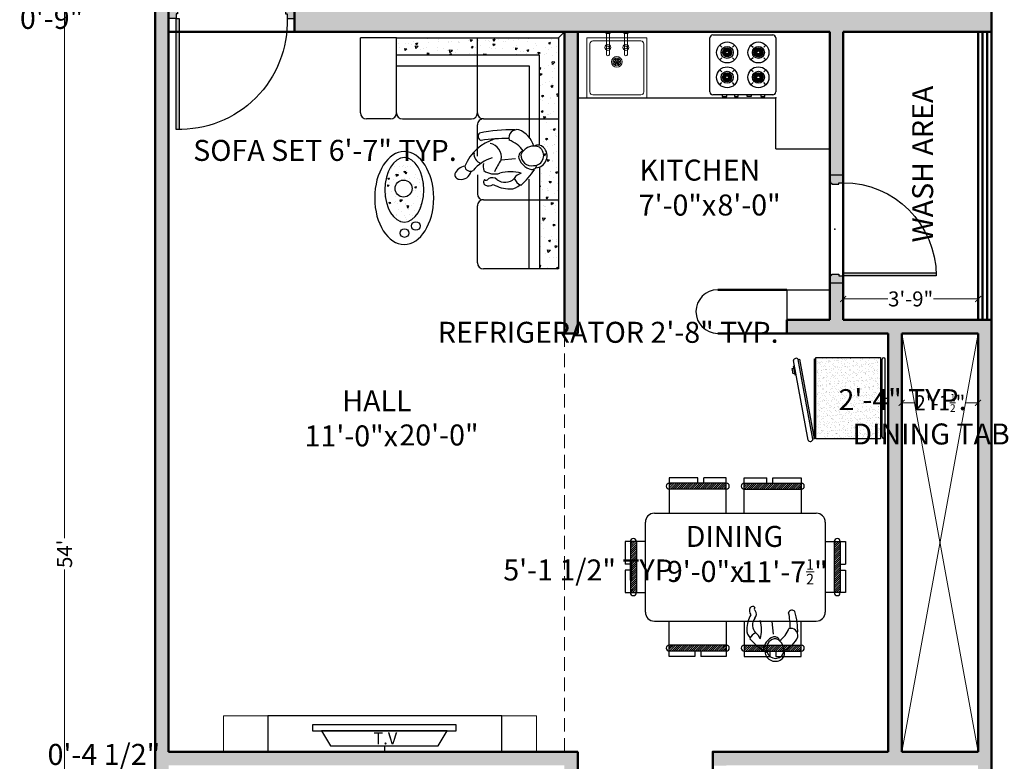
# Model space of a CAD drawing. Units: inches. Extents: x 4508 to 5907, y 877 to 1592.
# Tile 5 of 20: x 4874 to 5203, y 1182 to 1429. Entities that reach past the tile are written whole.
import ezdxf

# ---------------------------------------------------------------- set-up
doc = ezdxf.new("R2010")
doc.units = ezdxf.units.IN
doc.linetypes.add('DASHED', pattern=[0.75, 0.5, -0.25])
doc.layers.get('DEFPOINTS').update_dxf_attribs({"color": 8})
for name, color, linetype, lineweight in [('A-ANNO-DIMS', 2, 'Continuous', 18), ('A-ANNO-TEXT', 7, 'Continuous', 25), ('A-DOOR', 4, 'Continuous', 25), ('A-FLOR-CASE', 30, 'Continuous', 25), ('A-FLOR-FIXT', 8, 'Continuous', 18), ('A-FLOR-OVHD', 5, 'DASHED', 18), ('A-FLOR-SHFT', 8, 'Continuous', 18), ('A-FURN', 24, 'Continuous', 18), ('A-WALL', 7, 'Continuous', 50), ('A-WALL-PATT', 8, 'Continuous', 13)]:
    doc.layers.add(name, color=color, linetype=linetype, lineweight=lineweight)
doc.layers.add('doors & windows', color=30, linetype='Continuous')
doc.layers.add('furniture', color=24, linetype='Continuous')
doc.styles.get("Standard").update_dxf_attribs({"font": 'arial.ttf'})
doc.dimstyles.new('details', dxfattribs={"dimtxt": 5, "dimasz": 2, "dimexe": 2, "dimexo": 3, "dimgap": 1, "dimtad": 0, "dimdec": 1, "dimzin": 0, "dimdsep": 46, "dimlunit": 4, "dimtxsty": 'Standard', "dimblk": 'ARCHTICK', "dimcen": 3, "dimclrd": 256, "dimclre": 256, "dimclrt": 256, "dimadec": 0, "dimazin": 0, "dimtfac": 0.5, "dimtdec": 1, "dimtofl": 0, "dimtmove": 0, "dimatfit": 3, "dimldrblk": 'CLOSEDBLANK', "dimfxl": 2, "dimtolj": 1, "dimtzin": 0, "dimlwd": -1, "dimlwe": -1, "dimarcsym": 0})
doc.dimstyles.new('text', dxfattribs={"dimtxt": 7, "dimasz": 0, "dimexe": 3, "dimexo": 3, "dimgap": 0, "dimtad": 1, "dimtih": 1, "dimtoh": 1, "dimzin": 3, "dimdsep": 46, "dimlunit": 4, "dimtxsty": 'Standard', "dimblk": 'CLOSEDBLANK', "dimcen": 3, "dimse1": 1, "dimse2": 1, "dimsd1": 1, "dimsd2": 1, "dimclrd": 256, "dimclre": 256, "dimclrt": 256, "dimadec": 0, "dimazin": 0, "dimtfac": 0.5, "dimtofl": 0, "dimtmove": 0, "dimatfit": 3, "dimfxl": 3, "dimtolj": 1, "dimtzin": 0, "dimlwd": -1, "dimlwe": -1, "dimarcsym": 0})
pattern_1 = [(45, (0, 0), (-0.3535534, 0.3535534), [])]

# ---------------------------------------------------------------- blocks, each defined once
blk = doc.blocks.new('_ArchTick')
at = {"color": 0, "linetype": 'ByBlock', "const_width": 0.15}
blk.add_lwpolyline([(-0.5, -0.5), (0.5, 0.5)], dxfattribs=at)
blk = doc.blocks.new('*D52')
at = {"layer": 'A-ANNO-DIMS', "color": 0, "transparency": 16777216}
for p, q in [((4877.24, 1574.7), (4891.29, 1574.7)), ((4889.29, 1574.7), (4889.29, 1255.95)), ((4889.29, 926.7), (4889.29, 1245.46)), ((4877.24, 926.7), (4891.29, 926.7))]:
    blk.add_line(p, q, dxfattribs=at)
at = {"layer": 'DEFPOINTS', "color": 0, "transparency": 16777216}
for p in [(4874.24, 1574.7), (4874.24, 926.7), (4889.29, 926.7)]:
    blk.add_point(p, dxfattribs=at)
at = {"layer": 'A-ANNO-DIMS', "color": 0, "transparency": 16777216, "xscale": 2, "yscale": 2, "zscale": 2}
for p, rotation in [((4889.29, 1574.7), 90), ((4889.29, 926.7), 270)]:
    blk.add_blockref('_ArchTick', p, dxfattribs=dict(at, rotation=rotation))
at = {"layer": 'A-ANNO-DIMS', "color": 0, "transparency": 16777216, "insert": (4889.29, 1250.7), "char_height": 5, "attachment_point": 5, "rotation": 90}
blk.add_mtext("\\A1;54'", dxfattribs=at)
blk = doc.blocks.new('_ClosedBlank')
at = {"color": 0, "lineweight": -2}
for p, q in [((-1, 0.17), (0, 0)), ((-1, 0.17), (-1, -0.17)), ((0, 0), (-1, -0.17))]:
    blk.add_line(p, q, dxfattribs=at)
blk = doc.blocks.new('MD')
at = {"layer": 'doors & windows'}
h = blk.add_hatch(dxfattribs=at)
h.set_pattern_fill('DOTS', color=256, scale=2, style=0)
h.set_pattern_definition([(180, (0, -4), (-0.0625, 0.125), [0, -0.125])])
h.paths.add_polyline_path([(2.5, 37), (3.5, 37), (3.5, 0), (2.5, 0)])
h = blk.add_hatch(dxfattribs=at)
h.set_pattern_fill('DOTS', color=256, scale=2, style=0)
h.set_pattern_definition([(0, (0, -0.5), (0.0625, 0.125), [0, -0.125])])
h.paths.add_polyline_path([(42, -4.5), (42, 0), (39.5, 0), (39.5, -1.5), (39, -1.5), (39, -3.75), (39.25, -3.75, 0.403966), (39.75, -4.25), (39.75, -4.5)])
h.paths.add_polyline_path([(0, -4.5), (2.25, -4.5), (2.25, -4.25, 0.403966), (2.75, -3.75), (3, -3.75), (3, -1.5), (2.5, -1.5), (2.5, 0), (0, 0)])
for p, q in [((0, 0), (0, -4.5)), ((42, 0), (42, -4.5))]:
    blk.add_line(p, q)
blk.add_line((0, -4.5), (2.25, -4.5), dxfattribs=at)
blk.add_lwpolyline([(3.5, 0), (3.5, 37), (2.5, 37), (2.5, 0)], close=True, dxfattribs=at)
for points in [[(3, -3.75), (3, -1.5), (2.5, -1.5), (2.5, 0), (0, 0)], [(39, -3.75), (39, -1.5), (39.5, -1.5), (39.5, 0), (42, 0)], [(42, -4.5), (39.75, -4.5)]]:
    blk.add_lwpolyline(points, dxfattribs=at)
for points in [[(2.25, -4.5), (2.25, -4.25, 0.403966), (2.75, -3.75), (3, -3.75)], [(39.75, -4.5), (39.75, -4.25, -0.403966), (39.25, -3.75), (39, -3.75)]]:
    blk.add_lwpolyline(points, format="xyb", dxfattribs=at)
at = {"layer": 'doors & windows', "ltscale": 6}
blk.add_arc((3.73, 1.23), 35.79, 358.0281, 91.9719, dxfattribs=at)
at = {"layer": 'doors & windows'}
blk.add_point((21, -2.75), dxfattribs=at)
blk = doc.blocks.new('*D55')
at = {"layer": 'A-ANNO-DIMS', "color": 0, "transparency": 16777216}
for p, q in [((5148.99, 1331.7), (5148.99, 1337.68)), ((5193.99, 1331.7), (5193.99, 1337.68)), ((5148.99, 1335.68), (5163.85, 1335.68)), ((5193.99, 1335.68), (5179.14, 1335.68))]:
    blk.add_line(p, q, dxfattribs=at)
at = {"layer": 'DEFPOINTS', "color": 0, "transparency": 16777216}
for p in [(5193.99, 1335.68), (5148.99, 1328.7), (5193.99, 1328.7)]:
    blk.add_point(p, dxfattribs=at)
at = {"layer": 'A-ANNO-DIMS', "color": 0, "transparency": 16777216, "xscale": 2, "yscale": 2, "zscale": 2, "rotation": 180}
blk.add_blockref('_ArchTick', (5148.99, 1335.68), dxfattribs=at)
at = {"layer": 'A-ANNO-DIMS', "color": 0, "transparency": 16777216, "xscale": 2, "yscale": 2, "zscale": 2}
blk.add_blockref('_ArchTick', (5193.99, 1335.68), dxfattribs=at)
at = {"layer": 'A-ANNO-DIMS', "color": 0, "transparency": 16777216, "insert": (5171.49, 1335.68), "char_height": 5, "attachment_point": 5}
blk.add_mtext('\\A1;3\'-9"', dxfattribs=at)
blk = doc.blocks.new('D1')
at = {"layer": 'doors & windows'}
h = blk.add_hatch(dxfattribs=at)
h.set_pattern_fill('DOTS', color=256, scale=2, angle=180, style=0)
h.set_pattern_definition([(180, (-2e-12, -4), (-0.0625, -0.125), [0, -0.125])])
h.paths.add_polyline_path([(2.5, 0), (3.5, 0), (3.5, 30.98, 0.008066), (2.5, 31)])
h = blk.add_hatch(dxfattribs=at)
h.set_pattern_fill('DOTS', color=256, scale=2, angle=180, style=0)
h.set_pattern_definition([(180, (0, -0.5), (-0.0625, -0.125), [0, -0.125])])
h.paths.add_polyline_path([(0, -4.5), (2.25, -4.5), (2.25, -4.25, 0.403966), (2.75, -3.75), (3, -3.75), (3, -1.5), (2.5, -1.5), (2.5, 0), (0, 0)])
h.paths.add_polyline_path([(36, -4.5), (36, 0), (33.5, 0), (33.5, -1.5), (33, -1.5), (33, -3.75), (33.25, -3.75, 0.403966), (33.75, -4.25), (33.75, -4.5)])
for p, q in [((0, 0), (0, -4.5)), ((36, 0), (36, -4.5))]:
    blk.add_line(p, q)
blk.add_lwpolyline([(3.5, 0), (3.5, 31), (2.5, 31), (2.5, 0)], close=True, dxfattribs=at)
for points in [[(3, -3.75), (3, -1.5), (2.5, -1.5), (2.5, 0), (0, 0)], [(33, -3.75), (33, -1.5), (33.5, -1.5), (33.5, 0), (36, 0)], [(0, -4.5), (2.25, -4.5)], [(36, -4.5), (33.75, -4.5)]]:
    blk.add_lwpolyline(points, dxfattribs=at)
for points in [[(2.25, -4.5), (2.25, -4.25, 0.403966), (2.75, -3.75), (3, -3.75)], [(33.75, -4.5), (33.75, -4.25, -0.403966), (33.25, -3.75), (33, -3.75)]]:
    blk.add_lwpolyline(points, format="xyb", dxfattribs=at)
at = {"layer": 'doors & windows', "ltscale": 6}
blk.add_arc((2.5, 0), 31, 0, 90, dxfattribs=at)
at = {"layer": 'doors & windows'}
blk.add_point((18, -2.75), dxfattribs=at)
blk = doc.blocks.new('*D56')
at = {"layer": 'DEFPOINTS', "color": 0, "transparency": 16777216}
for p in [(5060.49, 1374.45), (5144.49, 1370.4), (5144.49, 1363.32)]:
    blk.add_point(p, dxfattribs=at)
at = {"layer": 'A-ANNO-DIMS', "color": 0, "transparency": 16777216, "insert": (5093.7, 1372.79), "char_height": 7, "attachment_point": 5}
blk.add_mtext('\\A1;       KITCHEN\\P7\'-0"x', dxfattribs=at)
blk = doc.blocks.new('*D57')
at = {"layer": 'DEFPOINTS', "color": 0, "transparency": 16777216}
for p in [(5099.76, 1424.7), (5117.58, 1424.7), (5125.91, 1328.7)]:
    blk.add_point(p, dxfattribs=at)
at = {"layer": 'A-ANNO-DIMS', "color": 0, "transparency": 16777216, "insert": (5117.58, 1367), "char_height": 7, "attachment_point": 5}
blk.add_mtext('\\A1;8\'-0"', dxfattribs=at)
blk = doc.blocks.new('stove')
at = {"layer": 'furniture'}
h = blk.add_hatch(dxfattribs=at)
h.set_pattern_fill('HEX', color=256, angle=180, style=0)
h.set_pattern_definition([(360, (22, 21.5), (1e-16, 0.2165064), [0.125, -0.25]), (120, (22, 21.5), (-0.1875, -0.1082532), [0.125, -0.25]), (60, (22.125, 21.5), (-0.1875, 0.1082532), [0.125, -0.25])])
h.paths.add_polyline_path([(5.36, 16.21, 1), (8.36, 16.21, 1)])
h.paths.add_polyline_path([(7.36, 16.21, -1), (6.36, 16.21, -1)], flags=16)
h = blk.add_hatch(dxfattribs=at)
h.set_pattern_fill('HEX', color=256, angle=180, style=0)
h.set_pattern_definition([(180, (2e-13, 21.5), (-1e-16, 0.2165064), [0.125, -0.25]), (60, (2e-13, 21.5), (0.1875, -0.1082532), [0.125, -0.25]), (120, (-0.125, 21.5), (0.1875, 0.1082532), [0.125, -0.25])])
h.paths.add_polyline_path([(13.64, 16.21, 1), (16.64, 16.21, 1)])
h.paths.add_polyline_path([(15.64, 16.21, -1), (14.64, 16.21, -1)], flags=16)
h = blk.add_hatch(dxfattribs=at)
h.set_pattern_fill('HEX', color=256, angle=180, style=0)
h.set_pattern_definition([(360, (22, 0.5), (-1e-16, -0.2165064), [0.125, -0.25]), (240, (22, 0.5), (-0.1875, 0.1082532), [0.125, -0.25]), (300, (22.125, 0.5), (-0.1875, -0.1082532), [0.125, -0.25])])
h.paths.add_polyline_path([(8.36, 5.79, 1), (5.36, 5.79, 1)])
h.paths.add_polyline_path([(6.36, 5.79, -1), (7.36, 5.79, -1)], flags=16)
h = blk.add_hatch(dxfattribs=at)
h.set_pattern_fill('HEX', color=256, angle=180, style=0)
h.set_pattern_definition([(180, (2e-13, 0.5), (1e-16, -0.2165064), [0.125, -0.25]), (300, (2e-13, 0.5), (0.1875, 0.1082532), [0.125, -0.25]), (240, (-0.125, 0.5), (0.1875, -0.1082532), [0.125, -0.25])])
h.paths.add_polyline_path([(16.64, 5.79, 1), (13.64, 5.79, 1)])
h.paths.add_polyline_path([(14.64, 5.79, -1), (15.64, 5.79, -1)], flags=16)
for p, q in [((1, 1), (1, 21)), ((2, 22), (20, 22)), ((21, 21), (21, 1)), ((1, 17.86), (0.5, 17.86)), ((0.5, 17.86), (0.5, 16.36)), ((4.39, 18.69), (5.1, 17.98)), ((8.63, 17.98), (9.34, 18.69)), ((13.37, 17.98), (12.66, 18.69)), ((17.61, 18.69), (16.9, 17.98)), ((0.5, 16.36), (1, 16.36)), ((0.5, 13.8), (0.5, 12.5)), ((1, 13.8), (0.5, 13.8)), ((4.39, 13.74), (5.1, 14.45)), ((8.63, 14.45), (9.34, 13.74)), ((13.37, 14.45), (12.66, 13.74)), ((17.61, 13.74), (16.9, 14.45)), ((0.5, 12.5), (1, 12.5)), ((0.5, 9.5), (1, 9.5)), ((0.5, 8.2), (0.5, 9.5)), ((1, 8.2), (0.5, 8.2)), ((4.39, 8.26), (5.1, 7.55)), ((8.63, 7.55), (9.34, 8.26)), ((13.37, 7.55), (12.66, 8.26)), ((17.61, 8.26), (16.9, 7.55)), ((0.5, 4.94), (0.5, 3.64)), ((1, 4.94), (0.5, 4.94)), ((0.5, 3.64), (1, 3.64)), ((4.39, 3.31), (5.1, 4.02)), ((8.63, 4.02), (9.34, 3.31)), ((13.37, 4.02), (12.66, 3.31)), ((17.61, 3.31), (16.9, 4.02)), ((20, 0), (2, 0))]:
    blk.add_line(p, q, dxfattribs=at)
for centre, radius in [((6.86, 16.21), 3.5), ((15.14, 16.21), 3.5), ((6.86, 16.21), 2), ((6.86, 16.21), 1.5), ((6.86, 16.21), 0.5), ((15.14, 16.21), 2), ((15.14, 16.21), 1.5), ((15.14, 16.21), 0.5), ((6.86, 5.79), 3.5), ((6.86, 5.79), 2), ((6.86, 5.79), 1.5), ((15.14, 5.79), 3.5), ((15.14, 5.79), 2), ((15.14, 5.79), 1.5), ((6.86, 5.79), 0.5), ((15.14, 5.79), 0.5)]:
    blk.add_circle(centre, radius, dxfattribs=at)
for centre, start, end in [((2, 21), 90, 180), ((20, 21), 0, 90), ((2, 1), 180, 270), ((20, 1), 270, 0)]:
    blk.add_arc(centre, 1, start, end, dxfattribs=at)
at = {"layer": 'furniture', "ltscale": 9}
blk.add_point((0, 0), dxfattribs=at)
blk = doc.blocks.new('sink')
for p, q in [((0, 0), (-24, 0)), ((0, 0), (0, 0)), ((-22, -3), (-2, -3)), ((-22, -23), (-22, -3)), ((-2, -3), (-2, -23)), ((-21, -21), (-21, -5)), ((-20, -4), (-4, -4)), ((-3, -5), (-3, -21)), ((-0.5, -9.5), (-7.5, -9.5)), ((-0.5, -9.5), (-0.5, -10.5)), ((0, -9), (0, -11)), ((-0.5, -10.5), (-7.5, -10.5)), ((-0.5, -15.5), (-7.5, -15.5)), ((-0.5, -15.5), (-0.5, -16.5)), ((0, -15), (0, -17)), ((-0.5, -16.5), (-7.5, -16.5)), ((-20, -22), (-4, -22)), ((-22, -23), (-2, -23))]:
    blk.add_line(p, q)
for centre, radius in [((-5.18, -10), 1), ((-5.18, -10), 0.5), ((-10, -13), 1.79), ((-10, -13), 1.29), ((-10.66, -12.62), 0.25), ((-10.66, -13.38), 0.25), ((-10, -12.24), 0.25), ((-10, -13), 0.25), ((-9.34, -12.62), 0.25), ((-9.34, -13.38), 0.25), ((-10, -13.76), 0.25), ((-5.18, -16), 1), ((-5.18, -16), 0.5)]:
    blk.add_circle(centre, radius)
for centre, radius, start, end in [((-20, -5), 1, 90, 180), ((-4, -5), 1, 0, 90), ((-7.5, -10), 0.5, 90, 270), ((0.01, -9.51), 0.511, 91.1728, 178.8272), ((0.01, -10.49), 0.511, 181.1728, 268.8272), ((-7.5, -16), 0.5, 90, 270), ((0.01, -15.51), 0.511, 91.1728, 178.8272), ((0.01, -16.49), 0.511, 181.1728, 268.8272), ((-20, -21), 1, 180, 270), ((-4, -21), 1, 270, 0)]:
    blk.add_arc(centre, radius, start, end)
blk = doc.blocks.new('*D58')
at = {"layer": 'A-ANNO-DIMS', "color": 0, "transparency": 16777216}
for p, q in [((5168.49, 1321.2), (5168.49, 1299.04)), ((5193.99, 1321.2), (5193.99, 1299.04)), ((5168.49, 1301.04), (5172.64, 1301.04)), ((5193.99, 1301.04), (5189.84, 1301.04))]:
    blk.add_line(p, q, dxfattribs=at)
at = {"layer": 'DEFPOINTS', "color": 0, "transparency": 16777216}
for p in [(5168.49, 1324.2), (5193.99, 1324.2), (5193.99, 1301.04)]:
    blk.add_point(p, dxfattribs=at)
at = {"layer": 'A-ANNO-DIMS', "color": 0, "transparency": 16777216, "xscale": 2, "yscale": 2, "zscale": 2, "rotation": 180}
blk.add_blockref('_ArchTick', (5168.49, 1301.04), dxfattribs=at)
at = {"layer": 'A-ANNO-DIMS', "color": 0, "transparency": 16777216, "xscale": 2, "yscale": 2, "zscale": 2}
blk.add_blockref('_ArchTick', (5193.99, 1301.04), dxfattribs=at)
at = {"layer": 'A-ANNO-DIMS', "color": 0, "transparency": 16777216, "insert": (5181.24, 1301.04), "char_height": 5, "attachment_point": 5}
blk.add_mtext('\\A1;2\'-1{\\H0.5x;\\S1/2;}"', dxfattribs=at)
blk = doc.blocks.new('refrigerator')
at = {"layer": 'furniture'}
h = blk.add_hatch(dxfattribs=at)
h.set_pattern_fill('AR-SAND', color=256, angle=-90, style=0)
h.set_pattern_definition([(307.5, (-13.5104, -1), (1.926824, 0.06299), [0, -1.52, 0, -1.7, 0, -1.625]), (277.5, (-13.5104, -1), (2.82215, -1.76978), [0, -0.82, 0, -1.37, 0, -0.525]), (237.5, (-13.5104, 0.23), (0.00566, -3.11414), [0, -0.5, 0, -1.8, 0, -2.35]), (227.5, (-13.5104, 0.23), (0.87768, -3.00613), [0, -0.25, 0, -1.18, 0, -1.35])])
h.paths.add_polyline_path([(13.6, -24.16), (13.6, -2.56), (-13.51, -2.56), (-13.51, -24.16)])
for p, q in [((0, -1), (0, 0)), ((-13.51, -2.56), (13.6, -2.56)), ((-13.51, -24.16), (-13.51, -2.56)), ((12.94, -1), (-12.94, -1)), ((12.94, -2), (-12.94, -2)), ((-12.41, -2), (-12.41, -2.56)), ((12.29, -2), (12.29, -2.56)), ((13.6, -2.56), (13.6, -24.16)), ((13.6, -24.16), (-13.51, -24.16)), ((-13.07, -24.59), (-13.07, -24.16)), ((13.26, -24.59), (-13.07, -24.59)), ((13.6, -24.61), (-12.95, -29.5)), ((13.7, -25.1), (-12.85, -29.99)), ((13.07, -24.59), (13.26, -24.62)), ((13.26, -24.62), (13.07, -24.71)), ((13.26, -24.59), (13.26, -24.16)), ((13.6, -24.61), (13.7, -25.1)), ((-12.85, -29.99), (-12.95, -29.5)), ((14.06, -26.73), (-12.49, -31.62)), ((-10.58, -31.27), (-10.49, -31.65)), ((-10.49, -31.65), (-7.79, -31.16)), ((-9.87, -32.01), (-9.97, -31.56)), ((-8.13, -31.69), (-9.87, -32.01)), ((-8.23, -31.24), (-8.13, -31.69)), ((-7.79, -31.16), (-7.88, -30.77))]:
    blk.add_line(p, q, dxfattribs=at)
for centre, radius, start, end in [((-12.94, -1.5), 0.5, 90, 270), ((12.94, -1.5), 0.5, 270, 90), ((13.58, -25.98), 0.888, 302.2332, 82.2568), ((-12.38, -30.74), 0.888, 122.2332, 262.2568)]:
    blk.add_arc(centre, radius, start, end, dxfattribs=at)
blk = doc.blocks.new('*D59')
at = {"layer": 'DEFPOINTS', "color": 0, "transparency": 16777216}
for p in [(5055.99, 1241.2), (5163.99, 1238.74), (5055.99, 1237.03)]:
    blk.add_point(p, dxfattribs=at)
at = {"layer": 'A-ANNO-DIMS', "color": 0, "transparency": 16777216, "insert": (5103.1, 1250.67), "char_height": 7, "attachment_point": 5}
blk.add_mtext('\\A1;         DINING\\P9\'-0"x', dxfattribs=at)
blk = doc.blocks.new('*D60')
at = {"layer": 'DEFPOINTS', "color": 0, "transparency": 16777216}
for p in [(5129.27, 1324.2), (5130.19, 1324.2), (5055.99, 1184.7)]:
    blk.add_point(p, dxfattribs=at)
at = {"layer": 'A-ANNO-DIMS', "color": 0, "transparency": 16777216, "insert": (5129.27, 1244.72), "char_height": 7, "attachment_point": 5}
blk.add_mtext('\\A1;11\'-7{\\H0.5x;\\S1/2;}"', dxfattribs=at)
blk = doc.blocks.new('DT')
at = {"layer": 'furniture'}
h = blk.add_hatch(dxfattribs=at)
h.set_pattern_fill('ANSI31', color=256, scale=4, style=0)
h.set_pattern_definition(pattern_1)
h.paths.add_polyline_path([(-34, -8.5), (-32, -8.5), (-32, 8.5), (-34, 8.5)])
h.paths.add_polyline_path([(-2, 26), (-2, 28), (-21, 28), (-21, 26)])
h.paths.add_polyline_path([(23, 26), (23, 28), (4, 28), (4, 26)])
h.paths.add_polyline_path([(23, -28), (23, -26), (4, -26), (4, -28)])
h.paths.add_polyline_path([(-2, -28), (-2, -26), (-21, -26), (-21, -28)])
h = blk.add_hatch(dxfattribs=at)
h.set_pattern_fill('ANSI31', color=256, scale=4, style=0)
h.set_pattern_definition(pattern_1)
h.paths.add_polyline_path([(34, -8.5), (36, -8.5), (36, 8.5), (34, 8.5)])
at = {"layer": 'doors & windows'}
blk.add_line((-11.2, 18.15), (-11.59, 22.33), dxfattribs=at)
for centre, radius, start, end in [((-13.21, 28.75), 2.25, 132.7993, 210.1219), ((-12.43, 27.51), 2.91, 359.7942, 144.0351), ((-12.34, 27.96), 3.42, 2.8928, 134.5528), ((-12.78, 20.33), 7.67, 108.0153, 157.5724), ((-11.2, 27.56), 3.95, 155.2349, 248.5051), ((-12.53, 26.93), 3.05, 267.7788, 10.6507), ((-13.37, 28.03), 5.08, 289.2819, 356.6237), ((-9.72, 27.09), 1.31, 352.7443, 87.7525), ((-20.97, 8.73), 22.84, 41.647, 56.3067), ((-17.49, 22.83), 2.42, 170.002, 284.7527), ((-8.5, 17.23), 8.99, 125.6851, 158.6987), ((-12.08, 24.9), 1.7, 192.3382, 283.0231), ((2.64, 20.82), 10.42, 162.7002, 196.7262), ((-4.27, 24.65), 3.12, 193.5598, 239.9446), ((-6.9, 24.92), 3.16, 289.6374, 341.2911), ((-6.62, 20.83), 3.81, 358.2671, 46.939), ((1.32, 21.08), 21.14, 177.1977, 197.248), ((6.61, 20.49), 23.98, 180.1725, 192.6992), ((-8.79, 19.27), 4.03, 325.4363, 41.8446), ((-13.17, 20.91), 10.36, 330.7562, 358.8997), ((-4.02, 15.59), 2.01, 136.0875, 215.1077), ((-17.93, 15.53), 1.19, 217.214, 345.0614), ((-5.98, 13.86), 0.655, 315.9836, 61.7947), ((-4.79, 14.1), 0.998, 224.0636, 323.687), ((-5.73, 14.57), 2.04, 328.4119, 38.6474)]:
    blk.add_arc(centre, radius, start, end, dxfattribs=at)
at = {"layer": 'furniture'}
for p, q in [((-21, 29.75), (-21, 18)), ((-12.5, 29.75), (-21, 29.75)), ((-12.5, 28), (-12.5, 29.75)), ((-10.5, 28), (-10.5, 29.75)), ((-2, 29.75), (-10.5, 29.75)), ((-2, 18), (-2, 29.75)), ((4, 18), (4, 29.75)), ((4, 29.75), (12.5, 29.75)), ((12.5, 28), (12.5, 29.75)), ((14.5, 28), (14.5, 29.75)), ((14.5, 29.75), (23, 29.75)), ((23, 29.75), (23, 18)), ((-2, 28), (-21, 28)), ((4, 28), (23, 28)), ((-2, 26), (-21, 26)), ((4, 26), (23, 26)), ((28, 18), (-26, 18)), ((-29, -15), (-29, 15)), ((31, 15), (31, -15)), ((-35.75, 1), (-35.75, 8.5)), ((-35.75, 8.5), (-29, 8.5)), ((-34, -8.5), (-34, 8.5)), ((-32, -8.5), (-32, 8.5)), ((37.75, 8.5), (31, 8.5)), ((34, -8.5), (34, 8.5)), ((36, -8.5), (36, 8.5)), ((37.75, 1), (37.75, 8.5)), ((-34, 1), (-35.75, 1)), ((36, 1), (37.75, 1)), ((-34, -1), (-35.75, -1)), ((-35.75, -8.5), (-35.75, -1)), ((36, -1), (37.75, -1)), ((37.75, -8.5), (37.75, -1)), ((-29, -8.5), (-35.75, -8.5)), ((31, -8.5), (37.75, -8.5)), ((28, -18), (-26, -18)), ((-21, -29.75), (-21, -18)), ((-2, -18), (-2, -29.75)), ((4, -18), (4, -29.75)), ((23, -29.75), (23, -18)), ((-2, -26), (-21, -26)), ((4, -26), (23, -26)), ((-2, -28), (-21, -28)), ((-11.5, -28), (-11.5, -29.75)), ((-9.5, -28), (-9.5, -29.75)), ((4, -28), (23, -28)), ((11.5, -28), (11.5, -29.75)), ((13.5, -28), (13.5, -29.75)), ((-11.5, -29.75), (-21, -29.75)), ((-2, -29.75), (-9.5, -29.75)), ((4, -29.75), (11.5, -29.75)), ((13.5, -29.75), (23, -29.75))]:
    blk.add_line(p, q, dxfattribs=at)
for centre, radius, start, end in [((-21, 27), 1, 90, 270), ((-2, 27), 1, 270, 90), ((4, 27), 1, 90, 270), ((23, 27), 1, 270, 90), ((-26, 15), 3, 90, 180), ((28, 15), 3, 0, 90), ((-33, 8.5), 1, 0, 180), ((35, 8.5), 1, 0, 180), ((-33, -8.5), 1, 180, 0), ((35, -8.5), 1, 180, 0), ((-26, -15), 3, 180, 270), ((28, -15), 3, 270, 0), ((-21, -27), 1, 90, 270), ((-2, -27), 1, 270, 90), ((4, -27), 1, 90, 270), ((23, -27), 1, 270, 90)]:
    blk.add_arc(centre, radius, start, end, dxfattribs=at)
blk.add_point((1, 0), dxfattribs=at)
blk = doc.blocks.new('tv')
at = {"layer": 'furniture'}
blk.add_line((0, 0), (2, 0), dxfattribs=at)
for points in [[(0, -39), (12, -39), (12, 39), (0, 39)], [(7, 24.19), (7, -23.81), (9, -23.81), (9, 24.19), (7, 24.19)]]:
    blk.add_lwpolyline(points, dxfattribs=at)
blk.add_lwpolyline([(7, -20.81), (7, 21.19), (2, 18.19), (2, -17.81)], close=True, dxfattribs=at)
blk.add_text('T.V', height=4, rotation=270, dxfattribs=at).set_placement((2.46, 3.81))
blk = doc.blocks.new('MAN')
at = {"layer": 'doors & windows'}
blk.add_line((1.3, -9.85), (0.89, -5.45), dxfattribs=at)
for centre, radius, start, end in [((-0.81, 1.3), 2.37, 132.7993, 210.1219), ((0, 0), 3.06, 359.7942, 144.0351), ((0.1, 0.48), 3.6, 2.8928, 134.5528), ((-0.36, -7.56), 8.07, 108.0153, 157.5724), ((1.3, 0.05), 4.16, 155.2349, 248.5051), ((-0.98, 0.55), 5.34, 289.2819, 356.6237), ((2.86, -0.44), 1.38, 352.7443, 87.7525), ((-8.99, -19.77), 24.04, 41.647, 56.3067), ((-0.1, -0.61), 3.22, 267.7788, 10.6507), ((-5.32, -4.92), 2.54, 170.002, 284.7527), ((34.75, -7.19), 42.53, 177.9613, 192.4551), ((4.14, -10.82), 9.46, 125.6851, 158.6987), ((0.38, -2.75), 1.79, 192.3382, 283.0231), ((15.87, -7.04), 10.97, 162.7002, 196.7262), ((8.59, -3.01), 3.29, 193.5598, 239.9446), ((5.83, -2.73), 3.32, 289.6374, 341.2911), ((3.84, -8.67), 4.24, 325.4363, 41.8446), ((6.12, -7.03), 4.01, 358.2671, 46.939), ((54.76, -7.35), 59.95, 180.1044, 188.2297), ((-0.78, -6.94), 10.91, 330.7562, 358.8997), ((9.03, -7.36), 14.72, 197.1765, 246.7641), ((0.5, -14.05), 4.27, 79.2575, 168.509), ((16.49, 13.41), 27.78, 236.8487, 245.427), ((-0.19, -11.81), 5.78, 325.2412, 16.1794), ((8.85, -12.54), 2.12, 136.0875, 215.1077), ((12.84, -8.62), 12.77, 197.9012, 229.3504), ((6.8, -14.37), 0.689, 315.9836, 61.7947), ((8.05, -14.12), 1.05, 224.0636, 323.687), ((7.06, -13.61), 2.15, 328.4119, 38.6474), ((-5.78, -15.61), 1.25, 217.214, 345.0614), ((-0.4, -15.27), 2.81, 261.6005, 345.5998), ((3.21, -8.72), 6.53, 262.8142, 281.931), ((3.09, -19.2), 1.68, 274.444, 31.8659), ((6.99, -20.36), 3.8, 187.9766, 248.0432), ((4.09, -22.01), 3.16, 349.15, 77.9716), ((5.75, -22.44), 1.45, 262.6631, 353.5986)]:
    blk.add_arc(centre, radius, start, end, dxfattribs=at)
blk = doc.blocks.new('sofa 3')
at = {"layer": 'furniture', "ltscale": 0.5}
h = blk.add_hatch(dxfattribs=at)
h.set_pattern_fill('AR-CONC', color=256, angle=90, style=0)
h.set_pattern_definition([(220, (1099.1507, -871.655), (0.627521, -7.172602), [0.75, -8.25]), (275, (1099.151, -871.655), (-7.52192, 1.387513), [0.6, -6.6]), (169.5486, (1099.203, -872.253), (-6.894395, -5.785094), [0.637402, -7.01142]), (223.8158, (1097.151, -871.655), (1.65519, -10.67241), [1.125, -12.375]), (173.3644, (1097.289, -872.544), (-9.74118, -9.34663), [0.9561, -10.51713]), (278.8158, (1097.151, -871.655), (-9.74119, -9.34662), [0.9, -9.9]), (249, (1097.6507, -872.655), (4.02619, -5.96907), [0.75, -8.25]), (304, (1097.651, -872.655), (-7.2515, -2.433153), [0.6, -6.6]), (198.5486, (1097.986, -873.1524), (-3.225305, -8.402226), [0.637402, -7.01142]), (232.5, (1099.1507, -871.655), (-3.3289385, -0.1215986), [0, -6.52, 0, -6.7, 0, -6.625]), (262.5, (1099.1507, -871.655), (-3.944117, -2.630695), [0, -3.82, 0, -6.37, 0, -2.525]), (302.5, (1099.1507, -869.425), (0.2255487, -5.3382244), [0, -2.5, 0, -7.8, 0, -10.35]), (312.5, (1099.1507, -868.425), (-1.00105, -5.831862), [0, -3.25, 0, -5.18, 0, -7.35])])
h.paths.add_polyline_path([(2, 56), (2, 79), (8.27, 79), (8.27, 56)])
edge = h.paths.add_edge_path()
edge.add_arc((9.44, 36.7), 1.54, 139.4115, 177.7525)
edge.add_arc((8.94, 33.52), 3.4, 107.8673, 234.0351)
edge.add_arc((8.88, 34.97), 4.62, 245.2349, 262.3616)
edge.add_line((8.27, 30.38), (8.27, 29))
edge.add_line((8.27, 29), (2, 29))
edge.add_line((2, 29), (2, 56))
edge.add_line((2, 56), (8.27, 56))
edge.add_line((8.27, 56), (8.27, 37.7))
h.paths.add_polyline_path([(8.27, 7.77), (29, 7.77), (29, 2), (2, 2), (2, 29), (8.27, 29)])
h.paths.add_polyline_path([(29, 2), (29, 7.77), (56, 7.77), (56, 2)])
at = {"layer": 'furniture'}
h = blk.add_hatch(dxfattribs=at)
h.set_pattern_fill('AR-CONC', color=256, scale=0.8, angle=90, style=0)
h.set_pattern_definition([(220, (892.888, -686.9864), (0.502017, -5.738081), [0.6, -6.6]), (275, (892.888, -686.9864), (-6.017537, 1.11001), [0.48, -5.28]), (169.5486, (892.93, -687.4646), (-5.515516, -4.628075), [0.509922, -5.609137]), (223.8158, (891.288, -686.9864), (1.32415, -8.53793), [0.9, -9.9]), (173.3644, (891.3985, -687.698), (-7.79294, -7.4773), [0.76488, -8.413704]), (278.8158, (891.288, -686.986), (-7.79295, -7.477296), [0.72, -7.92]), (249, (891.688, -687.7864), (3.220951, -4.775256), [0.6, -6.6]), (304, (891.688, -687.7864), (-5.8012, -1.946523), [0.48, -5.28]), (198.5486, (891.9566, -688.1844), (-2.580244, -6.72178), [0.509922, -5.609137]), (232.5, (892.8881, -686.9864), (-2.663151, -0.097279), [0, -5.216, 0, -5.36, 0, -5.3]), (262.5, (892.8881, -686.9864), (-3.155294, -2.104556), [0, -3.056, 0, -5.096, 0, -2.02]), (302.5, (892.8881, -685.2024), (0.180439, -4.2705795), [0, -2, 0, -6.24, 0, -8.28]), (312.5, (892.888, -684.4024), (-0.80084, -4.665489), [0, -2.6, 0, -4.144, 0, -5.88])])
edge = h.paths.add_edge_path()
edge.add_ellipse((53.37, 52.67), major_axis=(0, 10.76), ratio=0.60396, start_angle=0, end_angle=360, ccw=False)
h.paths.add_polyline_path([(56.46, 52.22, -1), (50.81, 52.22, -1)], flags=16)
for p, q in [((2, 2), (2, 79)), ((2, 79), (27, 79)), ((8.27, 44.99), (8.27, 79)), ((11.8, 79), (11.8, 49.12)), ((29, 77), (29, 58)), ((27, 56), (2, 56)), ((29, 47.65), (29, 54)), ((29, 41.41), (29, 31)), ((8.27, 37.77), (8.27, 7.77)), ((11.8, 11.29), (11.8, 35.08)), ((8.27, 29), (2, 29)), ((27, 29), (8.27, 29)), ((29, 27), (29, 2)), ((54, 29), (31, 29)), ((56, 27), (56, 2)), ((58, 29), (66, 29)), ((68, 27), (68, 2)), ((56, 11.29), (11.8, 11.29)), ((8.27, 7.77), (56, 7.77)), ((2, 2), (0, 0)), ((56, 2), (2, 2)), ((56, 2), (68, 2))]:
    blk.add_line(p, q, dxfattribs=at)
for centre, radius in [((49.58, 64.71), 1.44), ((53.36, 67.05), 1.44), ((53.63, 52.22), 2.83)]:
    blk.add_circle(centre, radius, dxfattribs=at)
for centre, start, end in [((27, 77), 0, 90), ((27, 58), 270, 0), ((27, 54), 0, 90), ((27, 31), 270, 0), ((27, 27), 0, 90), ((31, 27), 90, 180), ((54, 27), 0, 90), ((58, 27), 90, 180), ((66, 27), 0, 90)]:
    blk.add_arc(centre, 2, start, end, dxfattribs=at)
at = {"layer": 'furniture', "extrusion": (0, 0, -1)}
for centre, major_axis, ratio in [((53.43, 55.37), (0, 15.49), 0.635514), ((53.37, 52.67), (0, 10.76), 0.60396)]:
    blk.add_ellipse(centre, major_axis=major_axis, ratio=ratio, dxfattribs=at)
at = {"xscale": 1.1, "yscale": 1.1, "zscale": 1.1, "rotation": 90}
blk.add_blockref('MAN', (10.27, 41.21), dxfattribs=at)
blk = doc.blocks.new('*D71')
at = {"layer": 'DEFPOINTS', "color": 0, "transparency": 16777216}
for p in [(5002.43, 1422.87), (5014.16, 1422.87), (4995.88, 1182.87)]:
    blk.add_point(p, dxfattribs=at)
at = {"layer": 'A-ANNO-DIMS', "color": 0, "transparency": 16777216, "insert": (5014.16, 1290.32), "char_height": 7, "attachment_point": 5}
blk.add_mtext('\\A1;20\'-0"', dxfattribs=at)
blk = doc.blocks.new('*D72')
at = {"layer": 'DEFPOINTS', "color": 0, "transparency": 16777216}
for p in [(5063.81, 1286.44), (5063.81, 1261.14), (4931.81, 1252.3)]:
    blk.add_point(p, dxfattribs=at)
at = {"layer": 'A-ANNO-DIMS', "color": 0, "transparency": 16777216, "insert": (4984.91, 1295.85), "char_height": 7, "attachment_point": 5}
blk.add_mtext('\\A1;        HALL\\P11\'-0"x', dxfattribs=at)
blk = doc.blocks.new('*D77')
at = {"layer": 'A-ANNO-DIMS', "color": 0, "transparency": 16777216}
for p, q in [((5201.49, 1574.7), (5213.97, 1574.7)), ((5211.97, 1574.7), (5211.97, 1255.95)), ((5211.97, 926.7), (5211.97, 1245.46)), ((5201.49, 926.7), (5213.97, 926.7))]:
    blk.add_line(p, q, dxfattribs=at)
at = {"layer": 'DEFPOINTS', "color": 0, "transparency": 16777216}
for p in [(5198.49, 1574.7), (5211.97, 1574.7), (5198.49, 926.7)]:
    blk.add_point(p, dxfattribs=at)
at = {"layer": 'A-ANNO-DIMS', "color": 0, "transparency": 16777216, "xscale": 2, "yscale": 2, "zscale": 2}
for p, rotation in [((5211.97, 1574.7), 90), ((5211.97, 926.7), 270)]:
    blk.add_blockref('_ArchTick', p, dxfattribs=dict(at, rotation=rotation))
at = {"layer": 'A-ANNO-DIMS', "color": 0, "transparency": 16777216, "insert": (5211.97, 1250.7), "char_height": 5, "attachment_point": 5, "rotation": 90}
blk.add_mtext("\\A1;54'", dxfattribs=at)
blk = doc.blocks.new('*D168')
at = {"layer": 'DEFPOINTS', "color": 0, "transparency": 16777216}
for p in [(5163.99, 1320.93), (5131.98, 1316.12), (5163.99, 1316.12)]:
    blk.add_point(p, dxfattribs=at)
at = {"layer": 'A-ANNO-DIMS', "transparency": 16777216, "insert": (5070.62, 1324.55), "char_height": 7, "attachment_point": 5}
blk.add_mtext('\\A1;REFRIGERATOR 2\'-8" TYP.', dxfattribs=at)
blk = doc.blocks.new('*D169')
at = {"layer": 'DEFPOINTS', "color": 0, "transparency": 16777216}
for p in [(5163.99, 1316.12), (5163.99, 1288.08), (5168.79, 1288.08)]:
    blk.add_point(p, dxfattribs=at)
at = {"layer": 'A-ANNO-DIMS', "transparency": 16777216, "insert": (5168.79, 1302.1), "char_height": 7, "attachment_point": 5}
blk.add_mtext('\\A1;2\'-4" TYP.', dxfattribs=at)
blk = doc.blocks.new('*D170')
at = {"layer": 'DEFPOINTS', "color": 0, "transparency": 16777216}
for p in [(4987.99, 1424.7), (4976.14, 1345.7), (4987.99, 1345.7)]:
    blk.add_point(p, dxfattribs=at)
at = {"layer": 'A-ANNO-DIMS', "transparency": 16777216, "insert": (4976.14, 1385.2), "char_height": 7, "attachment_point": 5}
blk.add_mtext('\\A1;SOFA SET 6\'-7" TYP.', dxfattribs=at)
blk = doc.blocks.new('*D171')
at = {"layer": 'DEFPOINTS', "color": 0, "transparency": 16777216}
for p in [(4987.99, 1436.55), (4987.99, 1424.7), (5055.99, 1424.7)]:
    blk.add_point(p, dxfattribs=at)
at = {"layer": 'A-ANNO-DIMS', "transparency": 16777216, "insert": (5021.99, 1440.13), "char_height": 7, "attachment_point": 5}
blk.add_mtext('\\A1;5\'-8" TYP.', dxfattribs=at)
blk = doc.blocks.new('*D172')
at = {"layer": 'DEFPOINTS', "color": 0, "transparency": 16777216}
for p in [(5076.25, 1287.03), (5076.25, 1276.01), (5149.75, 1276.01)]:
    blk.add_point(p, dxfattribs=at)
at = {"layer": 'A-ANNO-DIMS', "transparency": 16777216, "insert": (5214.38, 1290.65), "char_height": 7, "attachment_point": 5}
blk.add_mtext('\\A1;DINING TABLE 6\'-1 1/2" TYP.', dxfattribs=at)
blk = doc.blocks.new('*D173')
at = {"layer": 'DEFPOINTS', "color": 0, "transparency": 16777216}
for p in [(5076.25, 1276.01), (5065.22, 1214.63), (5076.25, 1214.63)]:
    blk.add_point(p, dxfattribs=at)
at = {"layer": 'A-ANNO-DIMS', "transparency": 16777216, "insert": (5065.22, 1245.32), "char_height": 7, "attachment_point": 5}
blk.add_mtext('\\A1;5\'-1 1/2" TYP.', dxfattribs=at)
blk = doc.blocks.new('*D185')
at = {"layer": 'DEFPOINTS', "color": 0, "transparency": 16777216}
for p in [(4884.941772, 1433.703772), (4923.991772, 1433.703772), (4923.991772, 1424.703772)]:
    blk.add_point(p, dxfattribs=at)
at = {"layer": 'A-ANNO-DIMS', "transparency": 16777216, "insert": (4884.941772, 1429.203772), "char_height": 7, "attachment_point": 5}
blk.add_mtext('\\A1;0\'-9"', dxfattribs=at)
blk = doc.blocks.new('*D187')
at = {"layer": 'DEFPOINTS', "color": 0, "transparency": 16777216}
for p in [(4884.94, 1184.7), (4923.99, 1184.7), (4923.99, 1180.2)]:
    blk.add_point(p, dxfattribs=at)
at = {"layer": 'A-ANNO-DIMS', "transparency": 16777216, "insert": (4902.4, 1183.82), "char_height": 7, "attachment_point": 5}
blk.add_mtext('\\A1;0\'-4 1/2"', dxfattribs=at)

msp = doc.modelspace()

# ---------------------------------------------------------------- hatches: boundary and pattern name
at = {"layer": 'A-WALL-PATT'}
h = msp.add_hatch(color=256, dxfattribs=at)
h.dxf.hatch_style = 1
h.paths.add_polyline_path([(5198.492, 1496.704), (5108.492, 1496.704), (5108.492, 1473.841), (5117.492, 1473.841), (5117.492, 1487.704), (5189.492, 1487.704), (5189.492, 1433.704), (5117.492, 1433.704), (5117.492, 1442.024), (5115.492, 1442.024), (5108.492, 1442.024), (5108.492, 1433.704), (4965.992, 1433.704), (4965.992, 1424.704), (5144.492, 1424.704), (5144.492, 1376.919), (5148.992, 1376.919), (5148.992, 1424.704), (5198.492, 1424.704)])
h.paths.add_polyline_path([(5060.492, 1424.704), (5055.992, 1424.704), (5055.992, 1324.204), (5060.492, 1324.204)])
h = msp.add_hatch(color=256, dxfattribs=at)
h.dxf.hatch_style = 1
h.paths.add_polyline_path([(5198.492, 1328.704), (5148.992, 1328.704), (5148.992, 1340.919), (5144.492, 1340.919), (5144.492, 1328.704), (5130.194, 1328.704), (5130.194, 1324.204), (5163.992, 1324.204), (5163.992, 1184.704), (5105.492, 1184.704), (5105.492, 1180.124), (5109.992, 1180.124), (5109.992, 1180.204), (5193.992, 1180.204), (5193.992, 1115.704), (5109.992, 1115.704), (5109.992, 1123.704), (5109.992, 1150.124), (5105.492, 1150.124), (5105.492, 1115.704), (5096.492, 1115.704), (5096.492, 1111.204), (5193.992, 1111.204), (5193.992, 931.204), (5060.492, 931.204), (5060.492, 977.704), (5055.992, 977.704), (5055.992, 935.704), (5054.492, 935.704), (4983.992, 935.704), (4983.992, 1007.704), (4991.992, 1007.704), (5055.992, 1007.704), (5060.492, 1007.704), (5060.492, 1111.204), (5060.492, 1115.704), (5060.492, 1144.204), (5055.992, 1144.204), (5055.992, 1012.204), (4957.397, 1012.204), (4957.397, 1007.704), (4979.492, 1007.704), (4979.492, 926.704), (5198.492, 926.704)])
h.paths.add_polyline_path([(5193.992, 1184.704), (5168.492, 1184.704), (5168.492, 1324.204), (5193.992, 1324.204)], flags=16)
h.paths.add_polyline_path([(4923.992, 1180.204), (5055.992, 1180.204), (5055.992, 1144.204), (5060.492, 1144.204), (5060.492, 1184.704), (4923.992, 1184.704), (4923.992, 1424.704), (4923.992, 1433.704), (4919.492, 1433.704), (4919.492, 1007.704), (4957.397, 1007.704), (4957.397, 1012.204), (4923.992, 1012.204)])

# ---------------------------------------------------------------- linework, layer by layer
at = {"layer": 'A-FLOR-CASE'}
for p, q in [((5060.492, 1402.704), (5126.492, 1402.704)), ((5126.492, 1385.704), (5126.492, 1402.704)), ((5126.492, 1385.704), (5144.492, 1385.704)), ((5130.194, 1338.704), (5130.194, 1328.704))]:
    msp.add_line(p, q, dxfattribs=at)
msp.add_lwpolyline([(5130.194, 1338.704), (5144.492, 1338.704)], dxfattribs=at)
msp.add_arc((5107.128, 1331.454), 7.25, 90, 270, dxfattribs=at)
at = {"layer": 'A-FLOR-OVHD', "ltscale": 9}
msp.add_line((5055.992, 1324.204), (5055.992, 1184.704), dxfattribs=at)
at = {"layer": 'A-FLOR-SHFT', "ltscale": 9}
for p, q in [((5168.492, 1324.204), (5193.992, 1184.704)), ((5168.492, 1184.704), (5193.992, 1324.204))]:
    msp.add_line(p, q, dxfattribs=at)
at = {"layer": 'A-FURN'}
msp.add_lwpolyline([(5046.698, 1184.704), (5046.698, 1196.704), (4942.298, 1196.704), (4942.298, 1184.704)], dxfattribs=at)
at = {"layer": 'A-WALL'}
for p, q in [((4919.492, 926.704), (4919.492, 1574.704)), ((4923.992, 1424.704), (4923.992, 1574.704)), ((5198.492, 1574.704), (5198.492, 926.704)), ((4965.992, 1433.704), (4965.992, 1424.704)), ((4923.992, 1184.704), (4923.992, 1424.704)), ((4965.992, 1424.704), (4923.992, 1424.704)), ((5144.492, 1424.704), (4965.992, 1424.704)), ((5055.992, 1424.704), (5055.992, 1324.204)), ((5060.492, 1424.704), (5060.492, 1324.204)), ((5144.492, 1424.704), (5144.492, 1328.704)), ((5148.992, 1424.704), (5148.992, 1328.704)), ((5193.992, 1424.704), (5193.992, 1328.704)), ((5195.492, 1424.704), (5195.492, 1328.704)), ((5196.992, 1424.704), (5196.992, 1328.704)), ((5130.194, 1338.704), (5107.128, 1338.704)), ((5130.194, 1328.704), (5130.194, 1324.204)), ((5060.492, 1324.204), (5055.992, 1324.204)), ((5130.194, 1324.204), (5107.128, 1324.204)), ((5130.194, 1324.204), (5163.992, 1324.204)), ((5163.992, 1324.204), (5163.992, 1184.704)), ((5168.492, 1324.204), (5168.492, 1184.704)), ((5168.492, 1324.204), (5193.992, 1324.204)), ((5193.992, 1324.204), (5193.992, 1184.704)), ((4923.992, 1184.704), (5060.492, 1184.704)), ((5060.492, 1184.704), (5060.492, 1115.704))]:
    msp.add_line(p, q, dxfattribs=at)
for points in [[(5148.992, 1424.704), (5198.492, 1424.704)], [(5130.194, 1328.704), (5144.492, 1328.704)], [(5148.992, 1328.704), (5198.492, 1328.704)], [(5105.492, 1115.704), (5105.492, 1184.704), (5163.992, 1184.704)], [(5168.492, 1184.704), (5193.992, 1184.704)]]:
    msp.add_lwpolyline(points, dxfattribs=at)

# ---------------------------------------------------------------- block references
at = {"layer": 'A-DOOR', "xscale": -1}
for name, p, rotation in [('MD', (4923.992, 1429.204), 180), ('D1', (5148.992, 1340.919), 270)]:
    msp.add_blockref(name, p, dxfattribs=dict(at, rotation=rotation))
at = {"layer": 'A-FLOR-FIXT'}
for name, p, rotation in [('sink', (5060.492, 1424.704), 90), ('stove', (5126.492, 1402.704), 90), ('refrigerator', (5163.992, 1302.614), 270)]:
    msp.add_blockref(name, p, dxfattribs=dict(at, rotation=rotation))
at = {"layer": 'A-FURN'}
for name, p, rotation in [('sofa 3', (5055.992, 1424.704), 180), ('DT', (5113.996, 1246.259), 180), ('tv', (4996.127, 1184.704), 90)]:
    msp.add_blockref(name, p, dxfattribs=dict(at, rotation=rotation))

# ---------------------------------------------------------------- texts
at = {"layer": 'A-ANNO-TEXT'}
msp.add_text('WASH AREA', height=7, rotation=90, dxfattribs=at).set_placement((5178.996, 1354.503))

# ---------------------------------------------------------------- dimensions: what is measured, and where the dimension line sits
at = {"layer": 'A-ANNO-DIMS'}
for base, p1, p2, dimstyle, override, picture, middle in [((4889.286, 926.704), (4874.237, 1574.704), (4874.237, 926.704), 'details', {"dimclrd": 0, "dimclre": 0, "dimclrt": 0}, '*D52', (4889.286, 1250.704)), ((5211.971, 1574.704), (5198.492, 926.704), (5198.492, 1574.704), 'details', {"dimclrd": 0, "dimclre": 0, "dimclrt": 0}, '*D77', (5211.971, 1250.704)), ((4884.942, 1433.704), (4923.992, 1424.704), (4923.992, 1433.704), 'text', {"dimdec": 1, "dimlfac": 1, "dimrnd": 0, "dimzin": 1, "dimdsep": 46, "dimlunit": 4, "dimfrac": 2}, '*D185', (4884.942, 1429.204)), ((4884.942, 1184.704), (4923.992, 1180.204), (4923.992, 1184.704), 'text', {"dimdec": 1, "dimlfac": 1, "dimrnd": 0, "dimzin": 1, "dimdsep": 46, "dimlunit": 4, "dimfrac": 2}, '*D187', (4902.401, 1183.823))]:
    dim = msp.add_linear_dim(base=base, p1=p1, p2=p2, angle=90, dimstyle=dimstyle, override=override, dxfattribs=at)
    dim.commit()
    dim.dimension.update_dxf_attribs({"geometry": picture, "text_midpoint": middle})
for base, p1, p2, angle, text, picture, middle in [((4987.992, 1436.554), (5055.992, 1424.704), (4987.992, 1424.704), 180, '<> TYP.', '*D171', (5021.992, 1440.128)), ((4976.142, 1345.704), (4987.992, 1424.704), (4987.992, 1345.704), 270, 'SOFA SET <> TYP.', '*D170', (4976.142, 1385.204)), ((5076.246, 1287.034), (5149.746, 1276.009), (5076.246, 1276.009), 180, 'DINING TABLE <> TYP.', '*D172', (5214.381, 1290.653)), ((5168.793, 1288.084), (5163.992, 1316.124), (5163.992, 1288.084), 270, '<> TYP.', '*D169', (5168.793, 1302.104)), ((5065.221, 1214.625), (5076.246, 1276.009), (5076.246, 1214.625), 270, '<> TYP.', '*D173', (5065.221, 1245.317))]:
    dim = msp.add_linear_dim(base=base, p1=p1, p2=p2, angle=angle, text=text, dimstyle='text', override={"dimdec": 1, "dimrnd": 0, "dimzin": 1, "dimlunit": 4, "dimfrac": 2}, dxfattribs=at)
    dim.commit()
    dim.dimension.update_dxf_attribs({"geometry": picture, "text_midpoint": middle})
for base, p1, p2, picture, middle in [((5014.158, 1422.868), (4995.884, 1182.868), (5002.427, 1422.868), '*D71', (5014.158, 1290.324)), ((5117.576, 1424.704), (5125.91, 1328.704), (5099.756, 1424.704), '*D57', (5117.576, 1367.004)), ((5129.265, 1324.204), (5055.992, 1184.704), (5130.194, 1324.204), '*D60', (5129.265, 1244.723))]:
    dim = msp.add_linear_dim(base=base, p1=p1, p2=p2, angle=90, dimstyle='text', override={"dimclrd": 0, "dimclre": 0, "dimclrt": 0}, dxfattribs=at)
    dim.commit()
    dim.dimension.update_dxf_attribs({"geometry": picture, "text_midpoint": middle, "dimtype": 160})
for base, p1, p2, text, picture, middle in [((5144.492, 1363.324), (5060.492, 1374.454), (5144.492, 1370.398), '       KITCHEN\\P<>x', '*D56', (5093.701, 1363.324)), ((5063.811, 1286.439), (4931.811, 1252.298), (5063.811, 1261.141), '        HALL\\P<>x', '*D72', (4984.905, 1286.439))]:
    dim = msp.add_linear_dim(base=base, p1=p1, p2=p2, text=text, dimstyle='text', override={"dimclrd": 0, "dimclre": 0, "dimclrt": 0}, dxfattribs=at)
    dim.commit()
    dim.dimension.update_dxf_attribs({"geometry": picture, "text_midpoint": middle, "dimtype": 160})
dim = msp.add_linear_dim(base=(5163.992, 1320.926), p1=(5131.981, 1316.124), p2=(5163.992, 1316.124), text='REFRIGERATOR <> TYP.', dimstyle='text', override={"dimdec": 1, "dimrnd": 0, "dimzin": 1, "dimlunit": 4, "dimfrac": 2}, dxfattribs=at)
dim.commit()
dim.dimension.update_dxf_attribs({"geometry": '*D168', "text_midpoint": (5070.623, 1324.548)})
dim = msp.add_linear_dim(base=(5193.992, 1335.683), p1=(5148.992, 1328.704), p2=(5193.992, 1328.704), dimstyle='details', override={"dimclrd": 0, "dimclre": 0, "dimclrt": 0}, dxfattribs=at)
dim.commit()
dim.dimension.update_dxf_attribs({"geometry": '*D55', "text_midpoint": (5171.492, 1335.683), "dimtype": 160})
dim = msp.add_linear_dim(base=(5193.992, 1301.044), p1=(5168.492, 1324.204), p2=(5193.992, 1324.204), dimstyle='details', override={"dimclrd": 0, "dimclre": 0, "dimclrt": 0}, dxfattribs=at)
dim.commit()
dim.dimension.update_dxf_attribs({"geometry": '*D58', "text_midpoint": (5181.242, 1301.044)})
dim = msp.add_linear_dim(base=(5055.992, 1241.202), p1=(5163.992, 1238.745), p2=(5055.992, 1237.028), angle=180, text='         DINING\\P<>x', dimstyle='text', override={"dimclrd": 0, "dimclre": 0, "dimclrt": 0}, dxfattribs=at)
dim.commit()
dim.dimension.update_dxf_attribs({"geometry": '*D59', "text_midpoint": (5103.104, 1241.202), "dimtype": 160})

doc.saveas('drawing.dxf')
